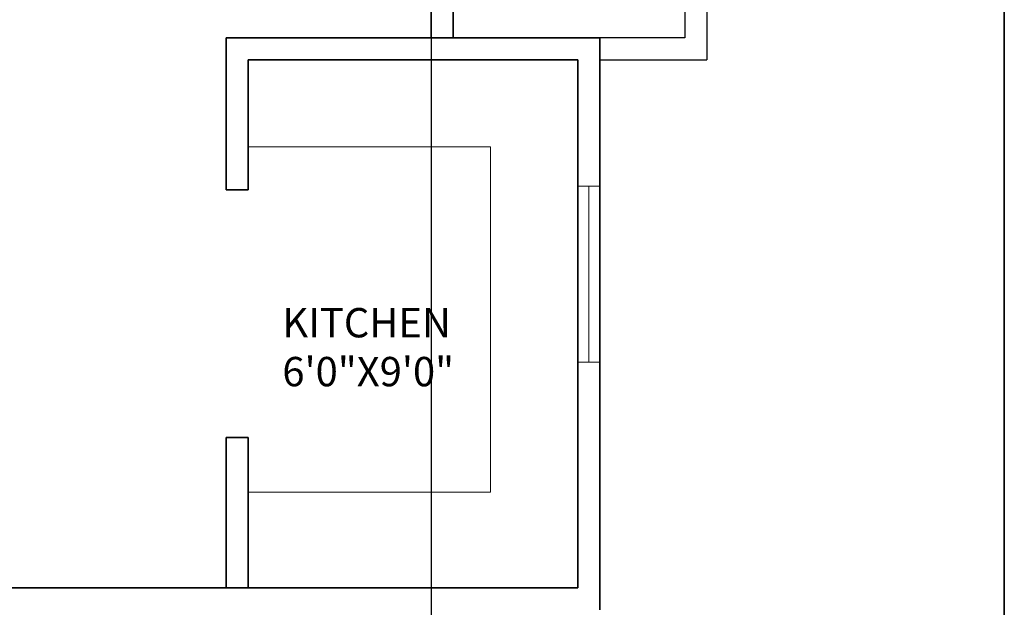
# Model space of a CAD drawing. Units: inches. Extents: x 1088 to 1703, y 668 to 1875.
# Tile 4 of 45: x 1502 to 1703, y 1069 to 1189. Entities that reach past the tile are written whole.
import ezdxf

# ---------------------------------------------------------------- set-up
doc = ezdxf.new("R2010")
doc.units = ezdxf.units.IN
for name, color, linetype, lineweight in [('A-ANNO-DIMS', 2, 'Continuous', 18), ('A-ANNO-TTLB', 7, 'Continuous', 35), ('A-AREA-IDEN', 7, 'Continuous', 18), ('A-FLOR-CASE', 8, 'Continuous', 18), ('A-FLOR-HRAL', 7, 'Continuous', 25), ('A-GLAZ', 4, 'Continuous', 18), ('A-WALL', 7, 'Continuous', 35)]:
    doc.layers.add(name, color=color, linetype=linetype, lineweight=lineweight)
doc.styles.get("Standard").update_dxf_attribs({"font": 'arial.ttf'})
doc.dimstyles.get("Standard").update_dxf_attribs({"dimtxt": 0.18, "dimasz": 0.18, "dimexe": 0.18, "dimexo": 0.0625, "dimgap": 0.09, "dimtad": 0, "dimtih": 1, "dimtoh": 1, "dimdec": 4, "dimzin": 0, "dimdsep": 46, "dimtxsty": 'Standard', "dimcen": 0.09, "dimadec": 0, "dimazin": 0, "dimtfac": 1, "dimtdec": 4, "dimtofl": 0, "dimtmove": 0, "dimatfit": 3, "dimfxl": 1, "dimtolj": 1, "dimtzin": 0, "dimarcsym": 0})

# ---------------------------------------------------------------- blocks, each defined once
blk = doc.blocks.new('WIN-36-RETURN')
for p, q in [((0, 36), (4.5, 36)), ((4.5, 36), (2.25, 36)), ((2.25, 36), (2.25, 0)), ((4.5, 0), (0, 0)), ((2.25, 0), (4.5, 0))]:
    blk.add_line(p, q)
blk = doc.blocks.new('*D31')
at = {"layer": 'A-ANNO-DIMS', "color": 0, "lineweight": -2, "transparency": 16777216}
for p, q in [((1435.84, 1326.5), (1435.84, 725.55)), ((1585.84, 1326.5), (1585.84, 725.55)), ((1436.02, 725.73), (1510.56, 725.73)), ((1585.66, 725.73), (1511.12, 725.73))]:
    blk.add_line(p, q, dxfattribs=at)
at = {"layer": 'A-ANNO-DIMS', "color": 0, "transparency": 16777216}
for points in [[(1436.02, 725.76), (1436.02, 725.7), (1435.84, 725.73)], [(1585.66, 725.76), (1585.66, 725.7), (1585.84, 725.73)]]:
    blk.add_solid(points, dxfattribs=at)
at = {"layer": 'Defpoints', "color": 0, "transparency": 16777216}
for p in [(1435.84, 1326.56), (1585.84, 1326.56), (1585.84, 725.73)]:
    blk.add_point(p, dxfattribs=at)
at = {"layer": 'A-ANNO-DIMS', "color": 0, "transparency": 16777216, "insert": (1510.84, 725.73), "char_height": 0.18, "attachment_point": 5}
blk.add_mtext('\\A1;150', dxfattribs=at)

msp = doc.modelspace()

# ---------------------------------------------------------------- linework, layer by layer
at = {"layer": 'A-ANNO-TTLB'}
msp.add_lwpolyline([(1088.369, 1874.677), (1703.181, 1874.677), (1703.181, 667.947), (1088.369, 667.947)], close=True, dxfattribs=at)
at = {"layer": 'A-FLOR-CASE'}
for p, q in [((1548.345, 1163.296), (1598.009, 1163.296)), ((1598.009, 1163.296), (1598.009, 1092.626)), ((1598.009, 1092.626), (1548.345, 1092.626))]:
    msp.add_line(p, q, dxfattribs=at)
at = {"layer": 'A-FLOR-HRAL'}
for p, q in [((1642.243, 1331.058), (1642.243, 1181.058)), ((1637.743, 1326.558), (1637.743, 1185.558)), ((1637.743, 1185.558), (1620.345, 1185.558)), ((1620.345, 1185.558), (1620.345, 1181.058)), ((1620.345, 1181.058), (1642.243, 1181.058))]:
    msp.add_line(p, q, dxfattribs=at)
at = {"layer": 'A-WALL'}
for p, q in [((1585.845, 1415.058), (1585.845, 1185.558)), ((1590.345, 1415.058), (1590.345, 1185.558)), ((1543.845, 1185.558), (1585.845, 1185.558)), ((1543.845, 1181.058), (1543.845, 1185.558)), ((1585.845, 1185.558), (1590.345, 1185.558)), ((1590.345, 1185.558), (1620.345, 1185.558)), ((1620.345, 1185.558), (1620.345, 1068.558)), ((1543.845, 1181.058), (1543.845, 1154.496)), ((1548.345, 1181.058), (1585.845, 1181.058)), ((1548.345, 1154.496), (1548.345, 1181.058)), ((1585.845, 1181.058), (1615.845, 1181.058)), ((1615.845, 1181.058), (1615.845, 1073.058)), ((1548.345, 1154.496), (1543.845, 1154.496)), ((1543.845, 1103.86), (1548.345, 1103.86)), ((1543.845, 1103.86), (1543.845, 1073.058)), ((1548.345, 1073.058), (1548.345, 1103.86)), ((1461.345, 1073.058), (1585.845, 1073.058)), ((1615.845, 1073.058), (1585.845, 1073.058))]:
    msp.add_line(p, q, dxfattribs=at)

# ---------------------------------------------------------------- block references
at = {"layer": 'A-GLAZ'}
msp.add_blockref('WIN-36-RETURN', (1615.845, 1119.221), dxfattribs=at)

# ---------------------------------------------------------------- texts
at = {"layer": 'A-AREA-IDEN', "insert": (1555.355, 1130.316), "char_height": 6, "attachment_point": 1}
msp.add_mtext_dynamic_manual_height_columns('KITCHEN\\P6\'0"X9\'0"', width=66.27691, gutter_width=12.5, heights=[0], dxfattribs=at)

# ---------------------------------------------------------------- dimensions: what is measured, and where the dimension line sits
at = {"layer": 'A-ANNO-DIMS'}
dim = msp.add_linear_dim(base=(1585.845, 725.729), p1=(1435.845, 1326.558), p2=(1585.845, 1326.558), dimstyle='Standard', override={"dimdec": 0, "dimlfac": 1, "dimrnd": 0, "dimzin": 0, "dimdsep": 46, "dimlunit": 2}, dxfattribs=at)
dim.commit()
dim.dimension.update_dxf_attribs({"geometry": '*D31', "text_midpoint": (1510.845, 725.729)})

doc.saveas('drawing.dxf')
